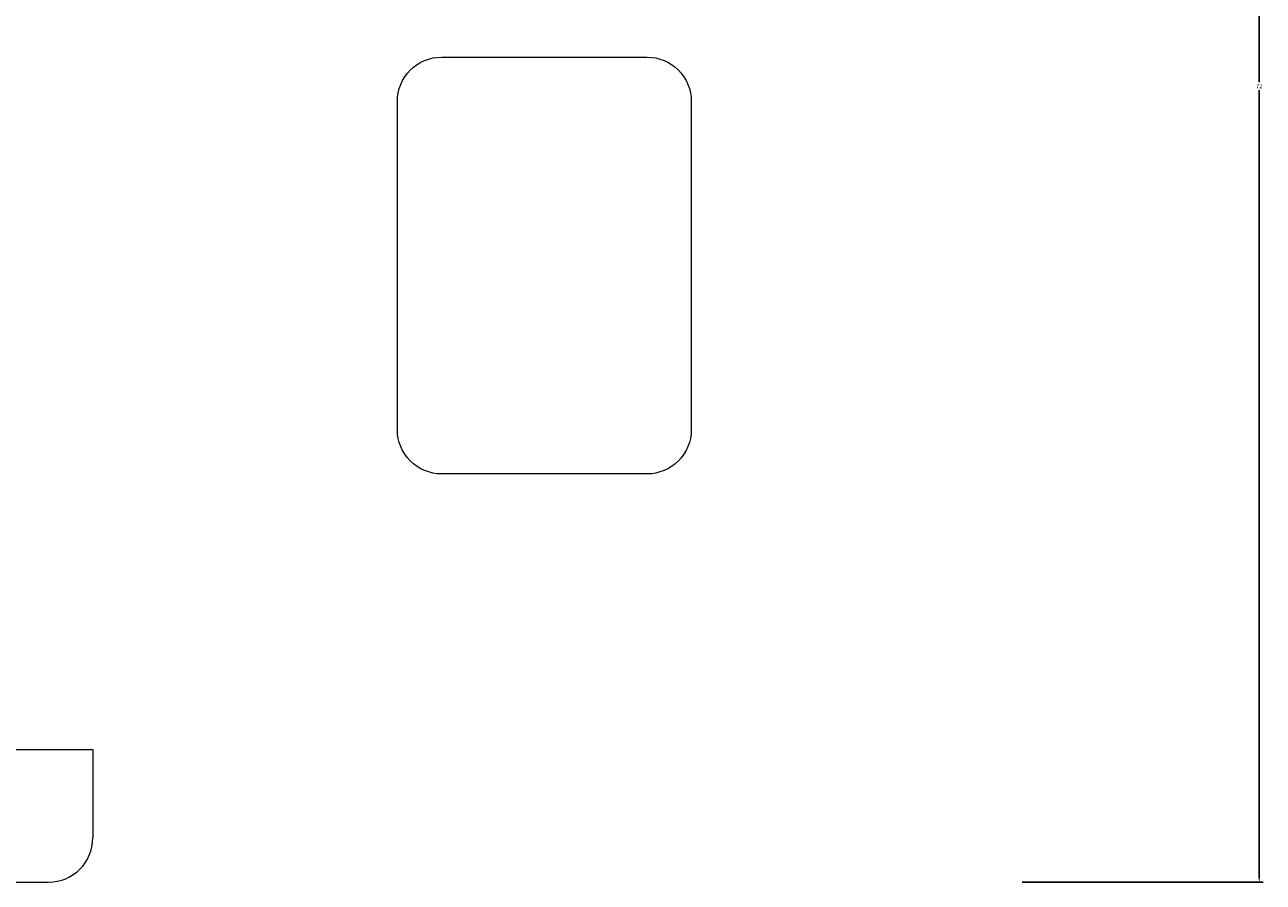
# Model space of a CAD drawing. Units: inches. Extents: x 2307 to 2544, y 2171 to 2540.
# Tile 3 of 52: x 2366 to 2422, y 2208 to 2247. Entities that reach past the tile are written whole.
import ezdxf

# ---------------------------------------------------------------- set-up
doc = ezdxf.new("R2010")
doc.units = ezdxf.units.IN
doc.layers.add('A-ANNO-DIMS', color=2, linetype='Continuous', lineweight=18)
doc.layers.add('A-FURN', color=8, linetype='Continuous', lineweight=18)
doc.styles.get("Standard").update_dxf_attribs({"font": 'arial.ttf'})
doc.dimstyles.get("Standard").update_dxf_attribs({"dimtxt": 0.18, "dimasz": 0.18, "dimexe": 0.18, "dimexo": 0.0625, "dimgap": 0.09, "dimtad": 0, "dimtih": 1, "dimtoh": 1, "dimdec": 4, "dimzin": 0, "dimdsep": 46, "dimtxsty": 'Standard', "dimcen": 0.09, "dimadec": 0, "dimazin": 0, "dimtfac": 1, "dimtdec": 4, "dimtofl": 0, "dimtmove": 0, "dimatfit": 3, "dimfxl": 1, "dimtolj": 1, "dimtzin": 0, "dimarcsym": 0})

# ---------------------------------------------------------------- blocks, each defined once
blk = doc.blocks.new('sofa')
for p, q in [((-15, -60), (9, -60)), ((9, -60), (9, -64)), ((-19, -66), (7, -66))]:
    blk.add_line(p, q)
blk.add_arc((7, -64), 2, 270, 0)
blk = doc.blocks.new('*D35')
at = {"layer": 'A-ANNO-DIMS', "color": 0, "lineweight": -2, "transparency": 16777216}
for p, q in [((2411.518, 2280.186), (2422.436, 2280.186)), ((2422.256, 2280.006), (2422.256, 2244.366)), ((2422.256, 2208.366), (2422.256, 2244.005)), ((2411.518, 2208.186), (2422.436, 2208.186))]:
    blk.add_line(p, q, dxfattribs=at)
at = {"layer": 'A-ANNO-DIMS', "color": 0, "transparency": 16777216}
for points in [[(2422.226, 2280.006), (2422.286, 2280.006), (2422.256, 2280.186)], [(2422.226, 2208.366), (2422.286, 2208.366), (2422.256, 2208.186)]]:
    blk.add_solid(points, dxfattribs=at)
at = {"layer": 'Defpoints', "color": 0, "transparency": 16777216}
for p in [(2411.456, 2280.186), (2422.256, 2280.186), (2411.456, 2208.186)]:
    blk.add_point(p, dxfattribs=at)
at = {"layer": 'A-ANNO-DIMS', "color": 0, "transparency": 16777216, "insert": (2422.256, 2244.186), "char_height": 0.18, "attachment_point": 5}
blk.add_mtext('\\A1;72', dxfattribs=at)

msp = doc.modelspace()

# ---------------------------------------------------------------- linework, layer by layer
at = {"layer": 'A-FURN'}
msp.add_lwpolyline([(2385.2423, 2245.5025), (2394.5466, 2245.5025, -0.4142136), (2396.5466, 2243.5025), (2396.5466, 2228.6531, -0.4142136), (2394.5466, 2226.6531), (2385.2423, 2226.6531, -0.4142136), (2383.2423, 2228.6531), (2383.2423, 2243.5025, -0.4142136)], format="xyb", close=True, dxfattribs=at)

# ---------------------------------------------------------------- block references
msp.add_blockref('sofa', (2360.4557, 2274.1858), dxfattribs=at)

# ---------------------------------------------------------------- dimensions: what is measured, and where the dimension line sits
at = {"layer": 'A-ANNO-DIMS'}
dim = msp.add_linear_dim(base=(2422.2557, 2280.1858), p1=(2411.4557, 2208.1858), p2=(2411.4557, 2280.1858), angle=90, dimstyle='Standard', override={"dimdec": 0, "dimlfac": 1, "dimrnd": 0, "dimzin": 0, "dimdsep": 46, "dimlunit": 2}, dxfattribs=at)
dim.commit()
dim.dimension.update_dxf_attribs({"geometry": '*D35', "text_midpoint": (2422.2557, 2244.1858)})

doc.saveas('drawing.dxf')
